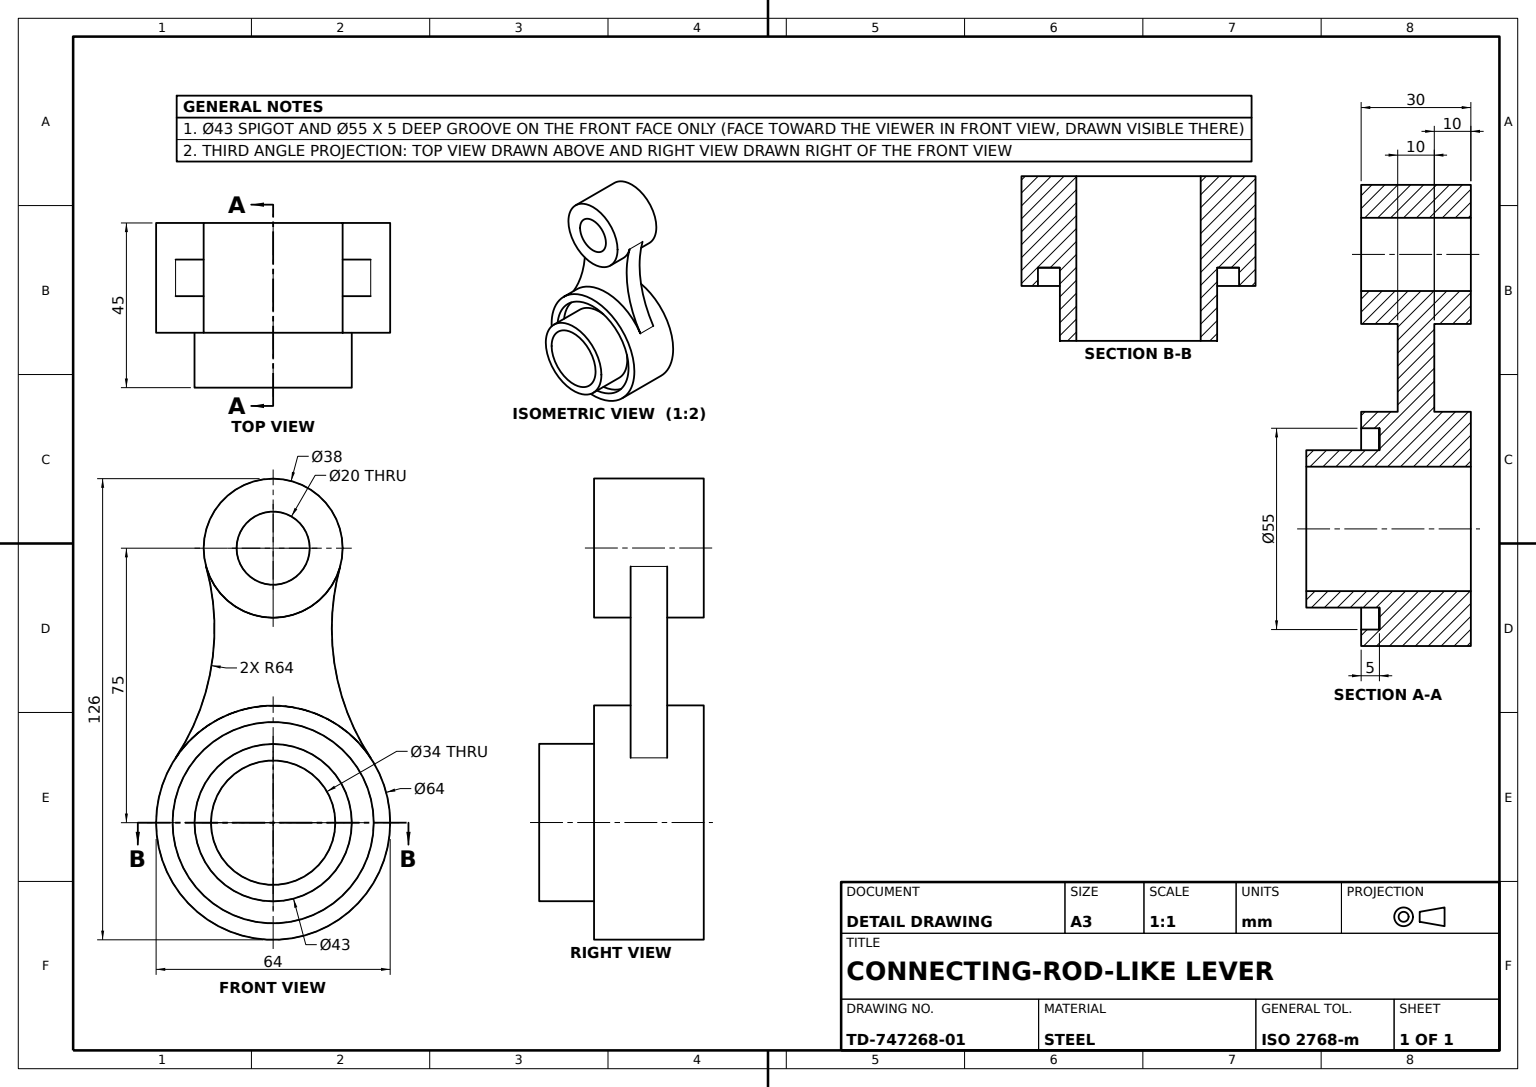
from build123d import *

# Parameters (mm, degrees)
LEVER_PROFILE_SKETCH_R         = 32
LEVER_PROFILE_SKETCH_R_2       = 27.5
LEVER_BODY_30MM_DEPTH          = 15
LEVER_PROFILE_SKETCH_R_3       = 19
LEVER_PROFILE_SKETCH_R_4       = 10
LEVER_BODY_30MM_2_DEPTH        = 15
WEB_EXTRUDE_10MM_DEPTH         = 5
BIG_END_HUB_10_15MM_DEPTH      = 10
BIG_END_HUB_10_15MM_DEPTH_BACK = 15
SKETCH1_5_R                    = 27.5
SKETCH1_5_R_2                  = 17
BIG_START                      = 10
SKETCH1_6_R                    = 21.5
SKETCH1_6_R_2                  = 17
BIG_END_SLEEVE_20MM_DEPTH      = 20


with BuildPart() as part:
    # Lever Profile Sketch → Lever Body 30mm (new, symmetric)
    with BuildSketch(Plane.XY):
        Circle(LEVER_PROFILE_SKETCH_R)
        Circle(LEVER_PROFILE_SKETCH_R_2, mode=Mode.SUBTRACT)
    extrude(amount=LEVER_BODY_30MM_DEPTH, both=True)



with BuildPart() as body_2:
    # Lever Profile Sketch → Lever Body 30mm 2 (new, symmetric)
    with BuildSketch(Plane.XY):
        with Locations((0, 75)):
            Circle(LEVER_PROFILE_SKETCH_R_3)
        with Locations((0, 75)):
            Circle(LEVER_PROFILE_SKETCH_R_4, mode=Mode.SUBTRACT)
    extrude(amount=LEVER_BODY_30MM_2_DEPTH, both=True)


with BuildPart() as part_1:
    add(part.part)

    add(body_2.part)  # Web Extrude 10mm merges body 2
    # Sketch1_4 → Web Extrude 10mm (add, symmetric)
    with BuildSketch(Plane.XY):
        with BuildLine():
            Line((0, 32), (0, 56))
            ThreePointArc((0, 56), (-11.518924537, 59.889924636), (-18.321243986, 69.966907631))
            ThreePointArc((-18.321243986, 69.966907631), (-16.836772686, 42.914041255), (-26.678302647, 17.671111111))
            ThreePointArc((-26.678302647, 17.671111111), (-15.141407538, 28.191093944), (0, 32))
        make_face()
        with BuildLine():
            ThreePointArc((18.321243986, 69.966907631), (11.518924537, 59.889924636), (0, 56))
            Line((0, 56), (0, 32))
            ThreePointArc((0, 32), (15.141407538, 28.191093944), (26.678302647, 17.671111111))
            ThreePointArc((26.678302647, 17.671111111), (16.836772686, 42.914041255), (18.321243986, 69.966907631))
        make_face()
    extrude(amount=WEB_EXTRUDE_10MM_DEPTH, both=True)

    # Sketch1_5 → Big End Hub 10_15mm (add, two sides: drawn at the far end of the back side and taken through both)
    with BuildSketch(Plane.XY.offset(-BIG_END_HUB_10_15MM_DEPTH_BACK)):
        Circle(SKETCH1_5_R)
        Circle(SKETCH1_5_R_2, mode=Mode.SUBTRACT)
    extrude(amount=BIG_END_HUB_10_15MM_DEPTH + BIG_END_HUB_10_15MM_DEPTH_BACK)

    # Sketch1_6 → Big End Sleeve 20mm (add)
    with BuildSketch(Plane.XY.offset(BIG_START)):
        Circle(SKETCH1_6_R)
        Circle(SKETCH1_6_R_2, mode=Mode.SUBTRACT)
    extrude(amount=BIG_END_SLEEVE_20MM_DEPTH)


solid = part_1.part
